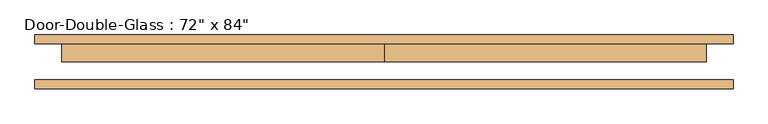
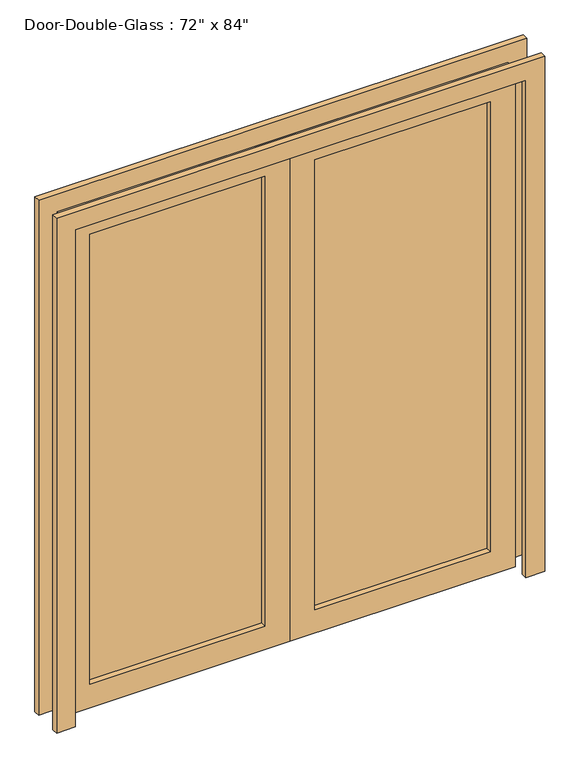
"""IFC4 building model written with IfcOpenShell, lengths in millimetres: door geometry."""

from ifc_helpers import new_model, si_unit, frame, origin, place, context, project, spatial, polyline, outline, extrude, source, transform, mapped, element, save


def door_8f551b21(model_context):
    return source(origin(), model_context, "Body", "SweptSolid", [
        extrude(outline(polyline([(2133.6, -914.4), (0.0, -914.4), (0.0, 0.0), (2133.6, 0.0), (2133.6, -914.4)]), holes=[polyline([(2032.0, -812.8), (2032.0, -101.6), (101.6, -101.6), (101.6, -812.8), (2032.0, -812.8)])]), frame((0.0, 2.38125, 0.0), z_axis=(0.0, 1.0, 0.0), x_axis=(0.0, 0.0, 1.0)), (0.0, 0.0, 1.0), 50.8),
        extrude(outline(polyline([(2133.6, 914.4), (2133.6, 0.0), (0.0, 0.0), (0.0, 914.4), (2133.6, 914.4)]), holes=[polyline([(2032.0, 812.8), (101.6, 812.8), (101.6, 101.6), (2032.0, 101.6), (2032.0, 812.8)])]), frame((0.0, 2.38125, 0.0), z_axis=(0.0, 1.0, 0.0), x_axis=(0.0, 0.0, 1.0)), (0.0, 0.0, 1.0), 50.8),
        extrude(outline(polyline([(101.6, 30.95625), (812.8, 30.95625), (812.8, 24.60625), (101.6, 24.60625), (101.6, 30.95625)])), frame((0.0, 0.0, 101.6), z_axis=(0.0, 0.0, 1.0), x_axis=(1.0, 0.0, 0.0)), (0.0, 0.0, 1.0), 1930.4),
        extrude(outline(polyline([(-812.8, 30.95625), (-101.6, 30.95625), (-101.6, 24.60625), (-812.8, 24.60625), (-812.8, 30.95625)])), frame((0.0, 0.0, 101.6), z_axis=(0.0, 0.0, 1.0), x_axis=(1.0, 0.0, 0.0)), (0.0, 0.0, 1.0), 1930.4),
        extrude(outline(polyline([(0.0, 990.6), (2209.8, 990.6), (2209.8, -990.6), (0.0, -990.6), (0.0, -914.4), (2133.6, -914.4), (2133.6, 914.4), (0.0, 914.4), (0.0, 990.6)])), frame((0.0, 53.18125, 0.0), z_axis=(0.0, 1.0, 0.0), x_axis=(0.0, 0.0, 1.0)), (0.0, 0.0, 1.0), 25.4),
        extrude(outline(polyline([(0.0, 990.6), (2209.8, 990.6), (2209.8, -990.6), (0.0, -990.6), (0.0, -914.4), (2133.6, -914.4), (2133.6, 914.4), (0.0, 914.4), (0.0, 990.6)])), frame((0.0, -73.81875, 0.0), z_axis=(0.0, 1.0, 0.0), x_axis=(0.0, 0.0, 1.0)), (0.0, 0.0, 1.0), 25.4),
    ])


if __name__ == "__main__":
    model = new_model("IFC4")
    model_context = context("Model", 3, world=origin())
    ifc_project = project(units=[si_unit("LENGTHUNIT", "METRE", prefix="MILLI")], contexts=[model_context])
    site = spatial("IfcSite", under=ifc_project)
    building = spatial("IfcBuilding", under=site)
    placement = place(None, origin())
    door_shape = door_8f551b21(model_context)
    element("IfcDoor", 1, ObjectType="Door-Double-Glass : 72\" x 84\"", at=placement, inside=building, context=model_context, shape_type="MappedRepresentation", body=[
        mapped(door_shape, transform((0.0, 0.0, 0.0), x_axis=(1.0, 0.0, 0.0), y_axis=(0.0, 1.0, 0.0), z_axis=(0.0, 0.0, 1.0))),
    ])
    save(model, "model.ifc")

# Revit data of these elements
# Type "Door-Double-Glass : 72\" x 84\""
#   Type Mark = "8"
#   Construction Type Id = "opn-d45"
#   Assembly Code = "C1020"
#   Analytic Construction = "Wood frame, double glass door "
#   W = 3' - 0"
#   Thickness = 0' - 2"
#   Thermal Resistance (R) = 1.8150 (h·ft²·°F)/BTU
#   Swing Angle [instance default] = 90.00°
#   Heat Transfer Coefficient (U) = 0.5510 BTU/(h·ft²·°F)
#   Height = 7' - 0"
#   Bottom Rail = 0' - 4"
#   Top Rail = 0' - 4"
#   Stiles = 0' - 4"
#   Trim Projection = 0' - 1"
#   Trim Width = 0' - 3"
#   Width = 6' - 0"
#   Define Thermal Properties by = 1
#   Glazing = Glass
#   Panel Material = Wood - Birch - Solid Stained Light Low Gloss
#   Trim Material = Paint - Sienna
#   Visual Light Transmittance = 0
#   Solar Heat Gain Coefficient = 0
#   Function = (empty or 0)
#   Wall Closure = (empty or 0)
# Element 1 (IfcDoor, "Door-Double-Glass : 72\" x 84\"")
#   Materials on its faces: "Wood - Birch - Solid Stained Light Low Gloss", "Paint - Sienna", "Glass"
# Materials
#   "Glass": class "Glass", colour RGB 0 128 192, transparency 0.75, Description = "Soda Lime Glass", Cost = 0
#   "Wood - Birch - Solid Stained Light Low Gloss": class "Wood", colour RGB 210 159 95, transparency 0, Cost = 0
#   "Paint - Sienna": colour RGB 118 70 51, transparency 0, Cost = 0
